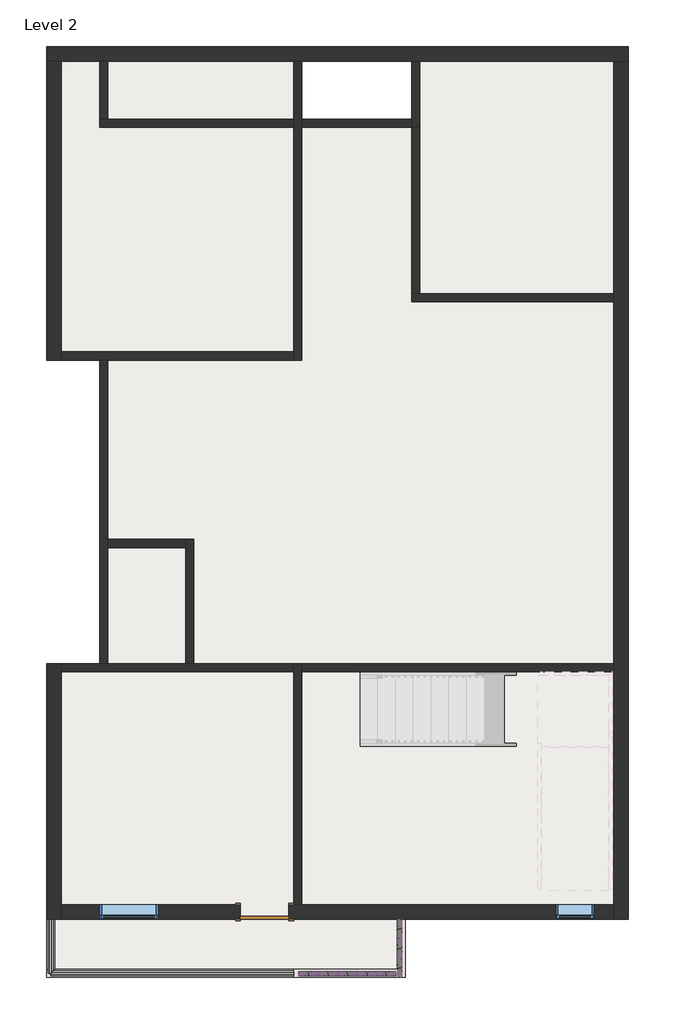
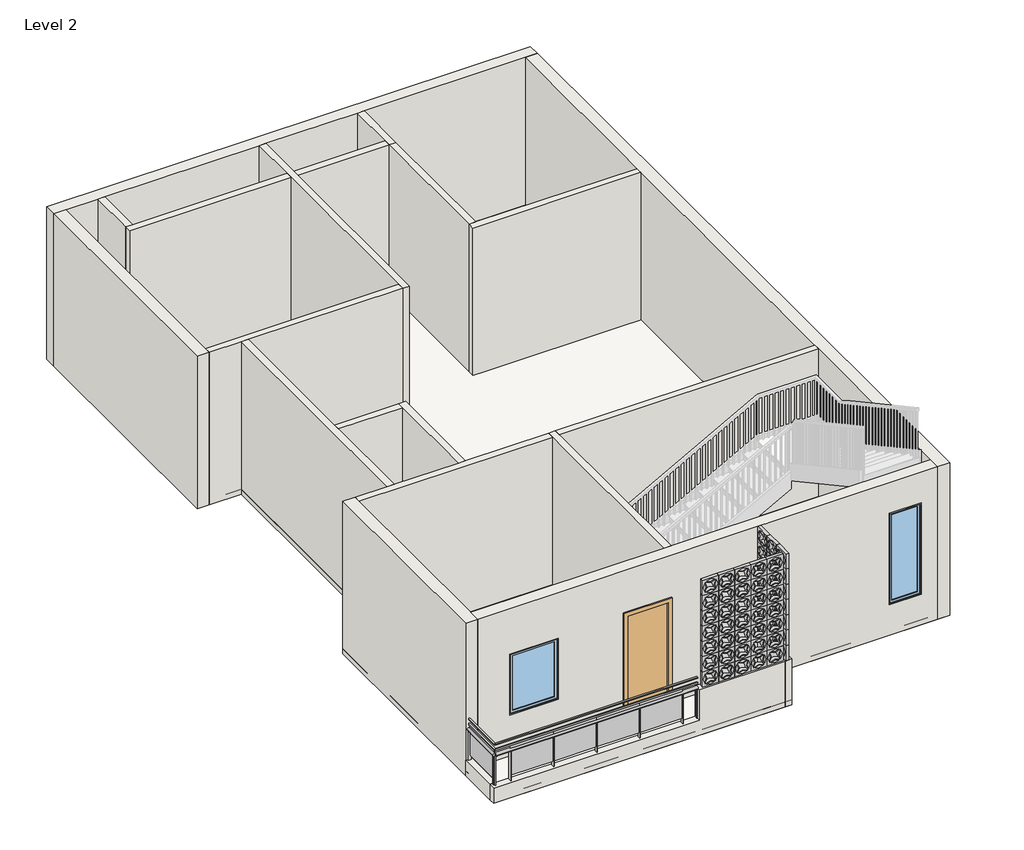
# One storey, part 1 of 2: 56 plates, 22 walls, 2 railings, 2 windows, 1 door, 1 roof.
"""IFC4 building model written with IfcOpenShell, lengths in millimetres."""

from ifc_helpers import new_model, si_unit, point, frame, origin, place, context, project, spatial, polyline, ellipse_curve, trimmed, outline, extrude, faceted_brep, transform, mapped, element, save
from ifc_brep_helpers import plane_surface, extruded_surface, advanced_brep
from components import door_5e1232af, plate_14329628, window_fc882ab3, fixed_4x3_c1f32544

model = new_model("IFC4")

# Units and contexts
model_context = context("Model", 3, world=origin())
ifc_project = project(units=[si_unit("LENGTHUNIT", "METRE", prefix="MILLI")], contexts=[model_context])

# Site, building, storey
site = spatial("IfcSite", under=ifc_project)
building = spatial("IfcBuilding", under=site)
storey = spatial("IfcBuildingStorey", under=building, Name="Level 2", Elevation=3048.0)

# Door
placement = place(None, origin())
door_shape = door_5e1232af(model_context)
element("IfcDoor", 1, ObjectType="Single-Flush : 30\" x 84\"", at=placement, inside=storey, context=model_context, shape_type="MappedRepresentation", body=[
    mapped(door_shape, transform((-1957.86646, -4503.4834702, 3048.0), x_axis=(1.0, 0.0, 0.0), y_axis=(0.0, 1.0, 0.0), z_axis=(0.0, 0.0, 1.0))),
])

# Plates
plate_shape = plate_14329628(model_context)
element("IfcPlate", 2, at=placement, inside=storey, context=model_context, shape_type="MappedRepresentation", body=[
    mapped(plate_shape, transform((194.78354, -4770.1834704, 3962.4), x_axis=(0.0, -1.0, 0.0), y_axis=(1.0, 0.0, 0.0), z_axis=(0.0, 0.0, 1.0))),
])
element("IfcPlate", 3, at=placement, inside=storey, context=model_context, shape_type="MappedRepresentation", body=[
    mapped(plate_shape, transform((194.78354, -5074.9834705, 3962.4), x_axis=(0.0, -1.0, 0.0), y_axis=(1.0, 0.0, 0.0), z_axis=(0.0, 0.0, 1.0))),
])
element("IfcPlate", 4, at=placement, inside=storey, context=model_context, shape_type="MappedRepresentation", body=[
    mapped(plate_shape, transform((194.78354, -5379.7834704, 3962.4), x_axis=(0.0, -1.0, 0.0), y_axis=(1.0, 0.0, 0.0), z_axis=(0.0, 0.0, 1.0))),
])
element("IfcPlate", 5, at=placement, inside=storey, context=model_context, shape_type="MappedRepresentation", body=[
    mapped(plate_shape, transform((194.78354, -4770.1834704, 4267.2), x_axis=(0.0, -1.0, 0.0), y_axis=(1.0, 0.0, 0.0), z_axis=(0.0, 0.0, 1.0))),
])
element("IfcPlate", 6, at=placement, inside=storey, context=model_context, shape_type="MappedRepresentation", body=[
    mapped(plate_shape, transform((194.78354, -5074.9834705, 4267.2), x_axis=(0.0, -1.0, 0.0), y_axis=(1.0, 0.0, 0.0), z_axis=(0.0, 0.0, 1.0))),
])
element("IfcPlate", 7, at=placement, inside=storey, context=model_context, shape_type="MappedRepresentation", body=[
    mapped(plate_shape, transform((194.78354, -5379.7834704, 4267.2), x_axis=(0.0, -1.0, 0.0), y_axis=(1.0, 0.0, 0.0), z_axis=(0.0, 0.0, 1.0))),
])
element("IfcPlate", 8, at=placement, inside=storey, context=model_context, shape_type="MappedRepresentation", body=[
    mapped(plate_shape, transform((194.78354, -4770.1834704, 4572.0), x_axis=(0.0, -1.0, 0.0), y_axis=(1.0, 0.0, 0.0), z_axis=(0.0, 0.0, 1.0))),
])
element("IfcPlate", 9, at=placement, inside=storey, context=model_context, shape_type="MappedRepresentation", body=[
    mapped(plate_shape, transform((194.78354, -5074.9834705, 4572.0), x_axis=(0.0, -1.0, 0.0), y_axis=(1.0, 0.0, 0.0), z_axis=(0.0, 0.0, 1.0))),
])
element("IfcPlate", 10, at=placement, inside=storey, context=model_context, shape_type="MappedRepresentation", body=[
    mapped(plate_shape, transform((194.78354, -5379.7834704, 4572.0), x_axis=(0.0, -1.0, 0.0), y_axis=(1.0, 0.0, 0.0), z_axis=(0.0, 0.0, 1.0))),
])
element("IfcPlate", 11, at=placement, inside=storey, context=model_context, shape_type="MappedRepresentation", body=[
    mapped(plate_shape, transform((194.78354, -4770.1834704, 4876.8), x_axis=(0.0, -1.0, 0.0), y_axis=(1.0, 0.0, 0.0), z_axis=(0.0, 0.0, 1.0))),
])
element("IfcPlate", 12, at=placement, inside=storey, context=model_context, shape_type="MappedRepresentation", body=[
    mapped(plate_shape, transform((194.78354, -5074.9834705, 4876.8), x_axis=(0.0, -1.0, 0.0), y_axis=(1.0, 0.0, 0.0), z_axis=(0.0, 0.0, 1.0))),
])
element("IfcPlate", 13, at=placement, inside=storey, context=model_context, shape_type="MappedRepresentation", body=[
    mapped(plate_shape, transform((194.78354, -5379.7834704, 4876.8), x_axis=(0.0, -1.0, 0.0), y_axis=(1.0, 0.0, 0.0), z_axis=(0.0, 0.0, 1.0))),
])
element("IfcPlate", 14, at=placement, inside=storey, context=model_context, shape_type="MappedRepresentation", body=[
    mapped(plate_shape, transform((194.78354, -4770.1834704, 5181.6), x_axis=(0.0, -1.0, 0.0), y_axis=(1.0, 0.0, 0.0), z_axis=(0.0, 0.0, 1.0))),
])
element("IfcPlate", 15, at=placement, inside=storey, context=model_context, shape_type="MappedRepresentation", body=[
    mapped(plate_shape, transform((194.78354, -5074.9834705, 5181.6), x_axis=(0.0, -1.0, 0.0), y_axis=(1.0, 0.0, 0.0), z_axis=(0.0, 0.0, 1.0))),
])
element("IfcPlate", 16, at=placement, inside=storey, context=model_context, shape_type="MappedRepresentation", body=[
    mapped(plate_shape, transform((194.78354, -5379.7834704, 5181.6), x_axis=(0.0, -1.0, 0.0), y_axis=(1.0, 0.0, 0.0), z_axis=(0.0, 0.0, 1.0))),
])
element("IfcPlate", 17, at=placement, inside=storey, context=model_context, shape_type="MappedRepresentation", body=[
    mapped(plate_shape, transform((194.78354, -4770.1834704, 5486.4), x_axis=(0.0, -1.0, 0.0), y_axis=(1.0, 0.0, 0.0), z_axis=(0.0, 0.0, 1.0))),
])
element("IfcPlate", 18, at=placement, inside=storey, context=model_context, shape_type="MappedRepresentation", body=[
    mapped(plate_shape, transform((194.78354, -5074.9834705, 5486.4), x_axis=(0.0, -1.0, 0.0), y_axis=(1.0, 0.0, 0.0), z_axis=(0.0, 0.0, 1.0))),
])
element("IfcPlate", 19, at=placement, inside=storey, context=model_context, shape_type="MappedRepresentation", body=[
    mapped(plate_shape, transform((194.78354, -5379.7834704, 5486.4), x_axis=(0.0, -1.0, 0.0), y_axis=(1.0, 0.0, 0.0), z_axis=(0.0, 0.0, 1.0))),
])
element("IfcPlate", 20, at=placement, inside=storey, context=model_context, shape_type="MappedRepresentation", body=[
    mapped(plate_shape, transform((194.78354, -4770.1834704, 5791.2), x_axis=(0.0, -1.0, 0.0), y_axis=(1.0, 0.0, 0.0), z_axis=(0.0, 0.0, 1.0))),
])
element("IfcPlate", 21, at=placement, inside=storey, context=model_context, shape_type="MappedRepresentation", body=[
    mapped(plate_shape, transform((194.78354, -5074.9834705, 5791.2), x_axis=(0.0, -1.0, 0.0), y_axis=(1.0, 0.0, 0.0), z_axis=(0.0, 0.0, 1.0))),
])
element("IfcPlate", 22, at=placement, inside=storey, context=model_context, shape_type="MappedRepresentation", body=[
    mapped(plate_shape, transform((194.78354, -5379.7834704, 5791.2), x_axis=(0.0, -1.0, 0.0), y_axis=(1.0, 0.0, 0.0), z_axis=(0.0, 0.0, 1.0))),
])
element("IfcPlate", 23, at=placement, inside=storey, context=model_context, shape_type="MappedRepresentation", body=[
    mapped(plate_shape, transform((-1272.0664598, -5443.2834702, 3962.4), x_axis=(1.0, 0.0, 0.0), y_axis=(0.0, 1.0, 0.0), z_axis=(0.0, 0.0, 1.0))),
])
element("IfcPlate", 24, at=placement, inside=storey, context=model_context, shape_type="MappedRepresentation", body=[
    mapped(plate_shape, transform((-967.2664597, -5443.2834702, 3962.4), x_axis=(1.0, 0.0, 0.0), y_axis=(0.0, 1.0, 0.0), z_axis=(0.0, 0.0, 1.0))),
])
element("IfcPlate", 25, at=placement, inside=storey, context=model_context, shape_type="MappedRepresentation", body=[
    mapped(plate_shape, transform((-662.4664597, -5443.2834702, 3962.4), x_axis=(1.0, 0.0, 0.0), y_axis=(0.0, 1.0, 0.0), z_axis=(0.0, 0.0, 1.0))),
])
element("IfcPlate", 26, at=placement, inside=storey, context=model_context, shape_type="MappedRepresentation", body=[
    mapped(plate_shape, transform((-1272.0664598, -5443.2834702, 4267.2), x_axis=(1.0, 0.0, 0.0), y_axis=(0.0, 1.0, 0.0), z_axis=(0.0, 0.0, 1.0))),
])
element("IfcPlate", 27, at=placement, inside=storey, context=model_context, shape_type="MappedRepresentation", body=[
    mapped(plate_shape, transform((-967.2664597, -5443.2834702, 4267.2), x_axis=(1.0, 0.0, 0.0), y_axis=(0.0, 1.0, 0.0), z_axis=(0.0, 0.0, 1.0))),
])
element("IfcPlate", 28, at=placement, inside=storey, context=model_context, shape_type="MappedRepresentation", body=[
    mapped(plate_shape, transform((-662.4664597, -5443.2834702, 4267.2), x_axis=(1.0, 0.0, 0.0), y_axis=(0.0, 1.0, 0.0), z_axis=(0.0, 0.0, 1.0))),
])
element("IfcPlate", 29, at=placement, inside=storey, context=model_context, shape_type="MappedRepresentation", body=[
    mapped(plate_shape, transform((-1272.0664598, -5443.2834702, 4572.0), x_axis=(1.0, 0.0, 0.0), y_axis=(0.0, 1.0, 0.0), z_axis=(0.0, 0.0, 1.0))),
])
element("IfcPlate", 30, at=placement, inside=storey, context=model_context, shape_type="MappedRepresentation", body=[
    mapped(plate_shape, transform((-967.2664597, -5443.2834702, 4572.0), x_axis=(1.0, 0.0, 0.0), y_axis=(0.0, 1.0, 0.0), z_axis=(0.0, 0.0, 1.0))),
])
element("IfcPlate", 31, at=placement, inside=storey, context=model_context, shape_type="MappedRepresentation", body=[
    mapped(plate_shape, transform((-662.4664597, -5443.2834702, 4572.0), x_axis=(1.0, 0.0, 0.0), y_axis=(0.0, 1.0, 0.0), z_axis=(0.0, 0.0, 1.0))),
])
element("IfcPlate", 32, at=placement, inside=storey, context=model_context, shape_type="MappedRepresentation", body=[
    mapped(plate_shape, transform((-1272.0664598, -5443.2834702, 4876.8), x_axis=(1.0, 0.0, 0.0), y_axis=(0.0, 1.0, 0.0), z_axis=(0.0, 0.0, 1.0))),
])
element("IfcPlate", 33, at=placement, inside=storey, context=model_context, shape_type="MappedRepresentation", body=[
    mapped(plate_shape, transform((-967.2664597, -5443.2834702, 4876.8), x_axis=(1.0, 0.0, 0.0), y_axis=(0.0, 1.0, 0.0), z_axis=(0.0, 0.0, 1.0))),
])
element("IfcPlate", 34, at=placement, inside=storey, context=model_context, shape_type="MappedRepresentation", body=[
    mapped(plate_shape, transform((-662.4664597, -5443.2834702, 4876.8), x_axis=(1.0, 0.0, 0.0), y_axis=(0.0, 1.0, 0.0), z_axis=(0.0, 0.0, 1.0))),
])
element("IfcPlate", 35, at=placement, inside=storey, context=model_context, shape_type="MappedRepresentation", body=[
    mapped(plate_shape, transform((-1272.0664598, -5443.2834702, 5181.6), x_axis=(1.0, 0.0, 0.0), y_axis=(0.0, 1.0, 0.0), z_axis=(0.0, 0.0, 1.0))),
])
element("IfcPlate", 36, at=placement, inside=storey, context=model_context, shape_type="MappedRepresentation", body=[
    mapped(plate_shape, transform((-967.2664597, -5443.2834702, 5181.6), x_axis=(1.0, 0.0, 0.0), y_axis=(0.0, 1.0, 0.0), z_axis=(0.0, 0.0, 1.0))),
])
element("IfcPlate", 37, at=placement, inside=storey, context=model_context, shape_type="MappedRepresentation", body=[
    mapped(plate_shape, transform((-662.4664597, -5443.2834702, 5181.6), x_axis=(1.0, 0.0, 0.0), y_axis=(0.0, 1.0, 0.0), z_axis=(0.0, 0.0, 1.0))),
])
element("IfcPlate", 38, at=placement, inside=storey, context=model_context, shape_type="MappedRepresentation", body=[
    mapped(plate_shape, transform((-1272.0664598, -5443.2834702, 5486.4), x_axis=(1.0, 0.0, 0.0), y_axis=(0.0, 1.0, 0.0), z_axis=(0.0, 0.0, 1.0))),
])
element("IfcPlate", 39, at=placement, inside=storey, context=model_context, shape_type="MappedRepresentation", body=[
    mapped(plate_shape, transform((-967.2664597, -5443.2834702, 5486.4), x_axis=(1.0, 0.0, 0.0), y_axis=(0.0, 1.0, 0.0), z_axis=(0.0, 0.0, 1.0))),
])
element("IfcPlate", 40, at=placement, inside=storey, context=model_context, shape_type="MappedRepresentation", body=[
    mapped(plate_shape, transform((-662.4664597, -5443.2834702, 5486.4), x_axis=(1.0, 0.0, 0.0), y_axis=(0.0, 1.0, 0.0), z_axis=(0.0, 0.0, 1.0))),
])
element("IfcPlate", 41, at=placement, inside=storey, context=model_context, shape_type="MappedRepresentation", body=[
    mapped(plate_shape, transform((-1272.0664598, -5443.2834702, 5791.2), x_axis=(1.0, 0.0, 0.0), y_axis=(0.0, 1.0, 0.0), z_axis=(0.0, 0.0, 1.0))),
])
element("IfcPlate", 42, at=placement, inside=storey, context=model_context, shape_type="MappedRepresentation", body=[
    mapped(plate_shape, transform((-967.2664597, -5443.2834702, 5791.2), x_axis=(1.0, 0.0, 0.0), y_axis=(0.0, 1.0, 0.0), z_axis=(0.0, 0.0, 1.0))),
])
element("IfcPlate", 43, at=placement, inside=storey, context=model_context, shape_type="MappedRepresentation", body=[
    mapped(plate_shape, transform((-662.4664597, -5443.2834702, 5791.2), x_axis=(1.0, 0.0, 0.0), y_axis=(0.0, 1.0, 0.0), z_axis=(0.0, 0.0, 1.0))),
])
element("IfcPlate", 44, at=placement, inside=storey, context=model_context, shape_type="MappedRepresentation", body=[
    mapped(plate_shape, transform((-357.6664597, -5443.2834702, 3962.4), x_axis=(1.0, 0.0, 0.0), y_axis=(0.0, 1.0, 0.0), z_axis=(0.0, 0.0, 1.0))),
])
element("IfcPlate", 45, at=placement, inside=storey, context=model_context, shape_type="MappedRepresentation", body=[
    mapped(plate_shape, transform((-357.6664597, -5443.2834702, 4267.2), x_axis=(1.0, 0.0, 0.0), y_axis=(0.0, 1.0, 0.0), z_axis=(0.0, 0.0, 1.0))),
])
element("IfcPlate", 46, at=placement, inside=storey, context=model_context, shape_type="MappedRepresentation", body=[
    mapped(plate_shape, transform((-357.6664597, -5443.2834702, 4572.0), x_axis=(1.0, 0.0, 0.0), y_axis=(0.0, 1.0, 0.0), z_axis=(0.0, 0.0, 1.0))),
])
element("IfcPlate", 47, at=placement, inside=storey, context=model_context, shape_type="MappedRepresentation", body=[
    mapped(plate_shape, transform((-357.6664597, -5443.2834702, 4876.8), x_axis=(1.0, 0.0, 0.0), y_axis=(0.0, 1.0, 0.0), z_axis=(0.0, 0.0, 1.0))),
])
element("IfcPlate", 48, at=placement, inside=storey, context=model_context, shape_type="MappedRepresentation", body=[
    mapped(plate_shape, transform((-357.6664597, -5443.2834702, 5181.6), x_axis=(1.0, 0.0, 0.0), y_axis=(0.0, 1.0, 0.0), z_axis=(0.0, 0.0, 1.0))),
])
element("IfcPlate", 49, at=placement, inside=storey, context=model_context, shape_type="MappedRepresentation", body=[
    mapped(plate_shape, transform((-357.6664597, -5443.2834702, 5486.4), x_axis=(1.0, 0.0, 0.0), y_axis=(0.0, 1.0, 0.0), z_axis=(0.0, 0.0, 1.0))),
])
element("IfcPlate", 50, at=placement, inside=storey, context=model_context, shape_type="MappedRepresentation", body=[
    mapped(plate_shape, transform((-357.6664597, -5443.2834702, 5791.2), x_axis=(1.0, 0.0, 0.0), y_axis=(0.0, 1.0, 0.0), z_axis=(0.0, 0.0, 1.0))),
])
element("IfcPlate", 51, at=placement, inside=storey, context=model_context, shape_type="MappedRepresentation", body=[
    mapped(plate_shape, transform((-52.8664598, -5443.2834702, 4267.2), x_axis=(1.0, 0.0, 0.0), y_axis=(0.0, 1.0, 0.0), z_axis=(0.0, 0.0, 1.0))),
])
element("IfcPlate", 52, at=placement, inside=storey, context=model_context, shape_type="MappedRepresentation", body=[
    mapped(plate_shape, transform((-52.8664598, -5443.2834702, 4572.0), x_axis=(1.0, 0.0, 0.0), y_axis=(0.0, 1.0, 0.0), z_axis=(0.0, 0.0, 1.0))),
])
element("IfcPlate", 53, at=placement, inside=storey, context=model_context, shape_type="MappedRepresentation", body=[
    mapped(plate_shape, transform((-52.8664598, -5443.2834702, 4876.8), x_axis=(1.0, 0.0, 0.0), y_axis=(0.0, 1.0, 0.0), z_axis=(0.0, 0.0, 1.0))),
])
element("IfcPlate", 54, at=placement, inside=storey, context=model_context, shape_type="MappedRepresentation", body=[
    mapped(plate_shape, transform((-52.8664598, -5443.2834702, 5791.2), x_axis=(1.0, 0.0, 0.0), y_axis=(0.0, 1.0, 0.0), z_axis=(0.0, 0.0, 1.0))),
])
element("IfcPlate", 55, at=placement, inside=storey, context=model_context, shape_type="MappedRepresentation", body=[
    mapped(plate_shape, transform((-52.8664598, -5443.2834702, 3962.4), x_axis=(1.0, 0.0, 0.0), y_axis=(0.0, 1.0, 0.0), z_axis=(0.0, 0.0, 1.0))),
])
element("IfcPlate", 56, at=placement, inside=storey, context=model_context, shape_type="MappedRepresentation", body=[
    mapped(plate_shape, transform((-52.8664598, -5443.2834702, 5181.6), x_axis=(1.0, 0.0, 0.0), y_axis=(0.0, 1.0, 0.0), z_axis=(0.0, 0.0, 1.0))),
])
element("IfcPlate", 57, at=placement, inside=storey, context=model_context, shape_type="MappedRepresentation", body=[
    mapped(plate_shape, transform((-52.8664598, -5443.2834702, 5486.4), x_axis=(1.0, 0.0, 0.0), y_axis=(0.0, 1.0, 0.0), z_axis=(0.0, 0.0, 1.0))),
])

# Railings
element("IfcRailing", 58, ObjectType="Glass Panel - Bottom Fill", at=placement, inside=storey, context=model_context, shape_type="SolidModel", body=[
    advanced_brep(
    [(-5285.26646, -4617.7834702, 3962.4), (-5361.46646, -4617.7834702, 3962.4), (-5285.26646, -5468.6834702, 3962.4), (-5361.46646, -5468.6834702, 3962.4)],
    [
        (0, 1, ellipse_curve(frame((-5323.36646, -4617.7834702, 3962.4), z_axis=(0.0, 1.0, 0.0), x_axis=(-1.0, 0.0, 0.0)), 38.1, 28.575)),
        (1, 0, ellipse_curve(frame((-5323.36646, -4617.7834702, 3962.4), z_axis=(0.0, 1.0, 0.0), x_axis=(-1.0, 0.0, 0.0)), 38.1, 28.575)),
        (2, 3, ellipse_curve(frame((-5323.36646, -5468.6834702, 3962.4), z_axis=(0.0, -1.0, 0.0), x_axis=(-1.0, 0.0, 0.0)), 38.1, 28.575)),
        (3, 2, ellipse_curve(frame((-5323.36646, -5468.6834702, 3962.4), z_axis=(0.0, -1.0, 0.0), x_axis=(-1.0, 0.0, 0.0)), 38.1, 28.575)),
        (0, 2),
        (3, 1),
    ],
    [
        plane_surface(frame((-5323.36646, -4617.7834702, 3962.4), z_axis=(0.0, 1.0, 0.0), x_axis=(0.0, 0.0, -1.0))),
        plane_surface(frame((-5323.36646, -5468.6834702, 3962.4), z_axis=(0.0, -1.0, 0.0), x_axis=(0.0, 0.0, -1.0))),
        extruded_surface(trimmed(ellipse_curve(frame((-5323.36646, -5468.6834702, 3962.4), z_axis=(0.0, 1.0, 0.0), x_axis=(-1.0, 0.0, 0.0)), 38.1, 28.575), [point((-5285.26646, -5468.6834702, 3962.4))], [point((-5361.46646, -5468.6834702, 3962.4))], True, "CARTESIAN"), (0.0, 850.8999999999996, 0.0), 850.8999999999996),
        extruded_surface(trimmed(ellipse_curve(frame((-5323.36646, -5468.6834702, 3962.4), z_axis=(0.0, 1.0, 0.0), x_axis=(-1.0, 0.0, 0.0)), 38.1, 28.575), [point((-5361.46646, -5468.6834702, 3962.4))], [point((-5285.26646, -5468.6834702, 3962.4))], True, "CARTESIAN"), (0.0, 850.8999999999996, 0.0), 850.8999999999996),
    ],
    [
        (0, [[1, 2]]),
        (1, [[3, 4]]),
        (2, [[-1, 5, -4, 6]]),
        (3, [[-2, -6, -3, -5]]),
    ],
),
    extrude(outline(polyline([(-5336.06646, -4617.7834702), (-5310.66646, -4617.7834702), (-5310.66646, -5468.6834702), (-5336.06646, -5468.6834702), (-5336.06646, -4617.7834702)])), frame((0.0, 0.0, 4152.9), z_axis=(0.0, 0.0, 1.0), x_axis=(1.0, 0.0, 0.0)), (0.0, 0.0, 1.0), 25.4),
    extrude(outline(polyline([(-5336.06646, -4617.7834702), (-5310.66646, -4617.7834702), (-5310.66646, -5468.6834702), (-5336.06646, -5468.6834702), (-5336.06646, -4617.7834702)])), frame((0.0, 0.0, 4051.3), z_axis=(0.0, 0.0, 1.0), x_axis=(1.0, 0.0, 0.0)), (0.0, 0.0, 1.0), 25.4),
    extrude(outline(polyline([(-5348.76646, -5443.2834702), (-5297.96646, -5443.2834702), (-5297.96646, -5455.9834702), (-5348.76646, -5455.9834702), (-5348.76646, -5443.2834702)])), frame((0.0, 0.0, 3352.8), z_axis=(0.0, 0.0, 1.0), x_axis=(1.0, 0.0, 0.0)), (0.0, 0.0, 1.0), 581.025),
    extrude(outline(polyline([(-5316.831303, -4636.8334702), (-5316.831303, -5449.6334702), (-5323.181303, -5449.6334702), (-5323.181303, -4636.8334702), (-5316.831303, -4636.8334702)])), frame((0.0, 0.0, 3454.4), z_axis=(0.0, 0.0, 1.0), x_axis=(1.0, 0.0, 0.0)), (0.0, 0.0, 1.0), 596.9),
    extrude(outline(polyline([(-5348.76646, -4630.4834702), (-5297.96646, -4630.4834702), (-5297.96646, -4643.1834702), (-5348.76646, -4643.1834702), (-5348.76646, -4630.4834702)])), frame((0.0, 0.0, 3352.8), z_axis=(0.0, 0.0, 1.0), x_axis=(1.0, 0.0, 0.0)), (0.0, 0.0, 1.0), 581.025),
    extrude(outline(polyline([(-5332.89146, -5455.9834702), (-5313.84146, -5455.9834702), (-5313.84146, -5475.0334702), (-5332.89146, -5475.0334702), (-5332.89146, -5455.9834702)])), frame((0.0, 0.0, 3352.8), z_axis=(0.0, 0.0, 1.0), x_axis=(1.0, 0.0, 0.0)), (0.0, 0.0, 1.0), 581.025),
    extrude(outline(polyline([(-5332.89146, -4611.4334702), (-5313.84146, -4611.4334702), (-5313.84146, -4630.4834702), (-5332.89146, -4630.4834702), (-5332.89146, -4611.4334702)])), frame((0.0, 0.0, 3352.8), z_axis=(0.0, 0.0, 1.0), x_axis=(1.0, 0.0, 0.0)), (0.0, 0.0, 1.0), 581.025),
])
element("IfcRailing", 59, ObjectType="Glass Panel - Bottom Fill", at=placement, inside=storey, context=model_context, shape_type="SolidModel", body=[
    advanced_brep(
    [(-1500.66646, -5506.7834702, 3962.4), (-1500.66646, -5430.5834702, 3962.4), (-5323.36646, -5506.7834702, 3962.4), (-5323.36646, -5430.5834702, 3962.4)],
    [
        (0, 1, ellipse_curve(frame((-1500.66646, -5468.6834702, 3962.4), z_axis=(1.0, 0.0, 0.0), x_axis=(0.0, 1.0, 0.0)), 38.1, 28.575)),
        (1, 0, ellipse_curve(frame((-1500.66646, -5468.6834702, 3962.4), z_axis=(1.0, 0.0, 0.0), x_axis=(0.0, 1.0, 0.0)), 38.1, 28.575)),
        (2, 3, ellipse_curve(frame((-5323.36646, -5468.6834702, 3962.4), z_axis=(-1.0, 0.0, 0.0), x_axis=(0.0, 1.0, 0.0)), 38.1, 28.575)),
        (3, 2, ellipse_curve(frame((-5323.36646, -5468.6834702, 3962.4), z_axis=(-1.0, 0.0, 0.0), x_axis=(0.0, 1.0, 0.0)), 38.1, 28.575)),
        (0, 2),
        (3, 1),
    ],
    [
        plane_surface(frame((-1500.66646, -5468.6834702, 3962.4), z_axis=(1.0, 0.0, 0.0), x_axis=(0.0, -1.0, 0.0))),
        plane_surface(frame((-5323.36646, -5468.6834702, 3962.4), z_axis=(-1.0, 0.0, 0.0), x_axis=(0.0, -1.0, 0.0))),
        extruded_surface(trimmed(ellipse_curve(frame((-5323.36646, -5468.6834702, 3962.4), z_axis=(1.0, 0.0, 0.0), x_axis=(0.0, 1.0, 0.0)), 38.1, 28.575), [point((-5323.36646, -5506.7834702, 3962.4))], [point((-5323.36646, -5430.5834702, 3962.4))], True, "CARTESIAN"), (3822.7000000000003, 0.0, 0.0), 3822.7000000000003),
        extruded_surface(trimmed(ellipse_curve(frame((-5323.36646, -5468.6834702, 3962.4), z_axis=(1.0, 0.0, 0.0), x_axis=(0.0, 1.0, 0.0)), 38.1, 28.575), [point((-5323.36646, -5430.5834702, 3962.4))], [point((-5323.36646, -5506.7834702, 3962.4))], True, "CARTESIAN"), (3822.7000000000003, 0.0, 0.0), 3822.7000000000003),
    ],
    [
        (0, [[1, 2]]),
        (1, [[3, 4]]),
        (2, [[-1, 5, -4, 6]]),
        (3, [[-2, -6, -3, -5]]),
    ],
),
    extrude(outline(polyline([(-1500.66646, -5455.9834702), (-1500.66646, -5481.3834702), (-5323.36646, -5481.3834702), (-5323.36646, -5455.9834702), (-1500.66646, -5455.9834702)])), frame((0.0, 0.0, 4152.9), z_axis=(0.0, 0.0, 1.0), x_axis=(1.0, 0.0, 0.0)), (0.0, 0.0, 1.0), 25.4),
    extrude(outline(polyline([(-1500.66646, -5455.9834702), (-1500.66646, -5481.3834702), (-5323.36646, -5481.3834702), (-5323.36646, -5455.9834702), (-1500.66646, -5455.9834702)])), frame((0.0, 0.0, 4051.3), z_axis=(0.0, 0.0, 1.0), x_axis=(1.0, 0.0, 0.0)), (0.0, 0.0, 1.0), 25.4),
    extrude(outline(polyline([(-5031.26646, -5443.2834702), (-5031.26646, -5494.0834702), (-5043.96646, -5494.0834702), (-5043.96646, -5443.2834702), (-5031.26646, -5443.2834702)])), frame((0.0, 0.0, 3352.8), z_axis=(0.0, 0.0, 1.0), x_axis=(1.0, 0.0, 0.0)), (0.0, 0.0, 1.0), 581.025),
    extrude(outline(polyline([(-4224.81646, -5475.2186272), (-5037.61646, -5475.2186272), (-5037.61646, -5468.8686272), (-4224.81646, -5468.8686272), (-4224.81646, -5475.2186272)])), frame((0.0, 0.0, 3454.4), z_axis=(0.0, 0.0, 1.0), x_axis=(1.0, 0.0, 0.0)), (0.0, 0.0, 1.0), 596.9),
    extrude(outline(polyline([(-4218.46646, -5443.2834702), (-4218.46646, -5494.0834702), (-4231.16646, -5494.0834702), (-4231.16646, -5443.2834702), (-4218.46646, -5443.2834702)])), frame((0.0, 0.0, 3352.8), z_axis=(0.0, 0.0, 1.0), x_axis=(1.0, 0.0, 0.0)), (0.0, 0.0, 1.0), 581.025),
    extrude(outline(polyline([(-3412.01646, -5475.2186272), (-4224.81646, -5475.2186272), (-4224.81646, -5468.8686272), (-3412.01646, -5468.8686272), (-3412.01646, -5475.2186272)])), frame((0.0, 0.0, 3454.4), z_axis=(0.0, 0.0, 1.0), x_axis=(1.0, 0.0, 0.0)), (0.0, 0.0, 1.0), 596.9),
    extrude(outline(polyline([(-3405.66646, -5443.2834702), (-3405.66646, -5494.0834702), (-3418.36646, -5494.0834702), (-3418.36646, -5443.2834702), (-3405.66646, -5443.2834702)])), frame((0.0, 0.0, 3352.8), z_axis=(0.0, 0.0, 1.0), x_axis=(1.0, 0.0, 0.0)), (0.0, 0.0, 1.0), 581.025),
    extrude(outline(polyline([(-2599.21646, -5475.2186272), (-3412.01646, -5475.2186272), (-3412.01646, -5468.8686272), (-2599.21646, -5468.8686272), (-2599.21646, -5475.2186272)])), frame((0.0, 0.0, 3454.4), z_axis=(0.0, 0.0, 1.0), x_axis=(1.0, 0.0, 0.0)), (0.0, 0.0, 1.0), 596.9),
    extrude(outline(polyline([(-2592.86646, -5443.2834702), (-2592.86646, -5494.0834702), (-2605.56646, -5494.0834702), (-2605.56646, -5443.2834702), (-2592.86646, -5443.2834702)])), frame((0.0, 0.0, 3352.8), z_axis=(0.0, 0.0, 1.0), x_axis=(1.0, 0.0, 0.0)), (0.0, 0.0, 1.0), 581.025),
    extrude(outline(polyline([(-1786.41646, -5475.2186272), (-2599.21646, -5475.2186272), (-2599.21646, -5468.8686272), (-1786.41646, -5468.8686272), (-1786.41646, -5475.2186272)])), frame((0.0, 0.0, 3454.4), z_axis=(0.0, 0.0, 1.0), x_axis=(1.0, 0.0, 0.0)), (0.0, 0.0, 1.0), 596.9),
    extrude(outline(polyline([(-1780.06646, -5443.2834702), (-1780.06646, -5494.0834702), (-1792.76646, -5494.0834702), (-1792.76646, -5443.2834702), (-1780.06646, -5443.2834702)])), frame((0.0, 0.0, 3352.8), z_axis=(0.0, 0.0, 1.0), x_axis=(1.0, 0.0, 0.0)), (0.0, 0.0, 1.0), 581.025),
    extrude(outline(polyline([(-5310.66646, -5459.1584702), (-5310.66646, -5478.2084702), (-5329.71646, -5478.2084702), (-5329.71646, -5459.1584702), (-5310.66646, -5459.1584702)])), frame((0.0, 0.0, 3352.8), z_axis=(0.0, 0.0, 1.0), x_axis=(1.0, 0.0, 0.0)), (0.0, 0.0, 1.0), 581.025),
    extrude(outline(polyline([(-1494.31646, -5459.1584702), (-1494.31646, -5478.2084702), (-1513.36646, -5478.2084702), (-1513.36646, -5459.1584702), (-1494.31646, -5459.1584702)])), frame((0.0, 0.0, 3352.8), z_axis=(0.0, 0.0, 1.0), x_axis=(1.0, 0.0, 0.0)), (0.0, 0.0, 1.0), 581.025),
])

# Roof
element("IfcRoof", 60, ObjectType="Generic - 4\"", at=placement, inside=storey, context=model_context, shape_type="Brep", body=[
    faceted_brep([(-5386.86646, 4170.6165298, 3048.0), (-5386.86646, 9098.2165298, 3048.0), (3757.13354, 9098.2165298, 3048.0), (3757.13354, -4617.7834702, 3048.0), (251.93354, -4617.7834702, 3048.0), (251.93354, -5532.1834702, 3048.0), (-5386.86646, -5532.1834702, 3048.0), (-5386.86646, -604.5834702, 3048.0), (-5158.26646, -604.5834702, 3048.0), (-4548.66646, -604.5834702, 3048.0), (-4548.66646, 4170.6165298, 3048.0), (-5158.26646, 4170.6165298, 3048.0), (353.53354, 8869.6165298, 3048.0), (-1373.66646, 8869.6165298, 3048.0), (-1373.66646, 7955.2165298, 3048.0), (353.53354, 7955.2165298, 3048.0), (3757.13354, -4617.7834702, 3149.6), (3757.13354, 9098.2165298, 3149.6), (-5386.86646, 9098.2165298, 3149.6), (-5386.86646, 4170.6165298, 3149.6), (-5158.26646, 4170.6165298, 3149.6), (-4548.66646, 4170.6165298, 3149.6), (-4548.66646, -604.5834702, 3149.6), (-5158.26646, -604.5834702, 3149.6), (-5386.86646, -604.5834702, 3149.6), (-5386.86646, -5532.1834702, 3149.6), (251.93354, -5532.1834702, 3149.6), (251.93354, -4617.7834702, 3149.6), (-1373.66646, 8869.6165298, 3149.6), (353.53354, 8869.6165298, 3149.6), (353.53354, 7955.2165298, 3149.6), (-1373.66646, 7955.2165298, 3149.6)], [[[0, 1, 2, 3, 4, 5, 6, 7, 8, 9, 10, 11], [12, 13, 14, 15]], [[16, 17, 18, 19, 20, 21, 22, 23, 24, 25, 26, 27], [28, 29, 30, 31]], [[2, 1, 18, 17]], [[1, 0, 19, 18]], [[3, 2, 17, 16]], [[4, 3, 16, 27]], [[5, 4, 27, 26]], [[6, 5, 26, 25]], [[12, 29, 28, 13]], [[13, 28, 31, 14]], [[14, 31, 30, 15]], [[29, 12, 15, 30]], [[22, 9, 8, 7, 24, 23]], [[10, 9, 22, 21]], [[19, 0, 11, 10, 21, 20]], [[7, 6, 25, 24]]]),
])

# Walls
element("IfcWall", 61, ObjectType="Generic - 5\"", at=placement, inside=storey, context=model_context, shape_type="Brep", body=[
    faceted_brep([(-1500.66646, -604.5834702, 3048.0), (-3075.46646, -604.5834702, 3048.0), (-3202.46646, -604.5834702, 3048.0), (-4421.66646, -604.5834702, 3048.0), (-4548.66646, -604.5834702, 3048.0), (-5158.26646, -604.5834702, 3048.0), (-5158.26646, -604.5834702, 6096.0), (-4548.66646, -604.5834702, 6096.0), (-4421.66646, -604.5834702, 6096.0), (-3202.46646, -604.5834702, 6096.0), (-3075.46646, -604.5834702, 6096.0), (-1500.66646, -604.5834702, 6096.0), (-1500.66646, -731.5834702, 3048.0), (-1500.66646, -731.5834702, 6096.0), (-5158.26646, -731.5834702, 6096.0), (-5158.26646, -731.5834702, 3048.0)], [[[0, 1, 2, 3, 4, 5, 6, 7, 8, 9, 10, 11]], [[12, 13, 14, 15]], [[5, 4, 3, 2, 1, 0, 12, 15]], [[11, 10, 9, 8, 7, 6, 14, 13]], [[0, 11, 13, 12]], [[6, 5, 15, 14]]]),
])
element("IfcWall", 62, ObjectType="Generic - 5\"", at=placement, inside=storey, context=model_context, shape_type="SweptSolid", body=[
    extrude(outline(polyline([(3528.53354, -731.5834702), (-1373.66646, -731.5834702), (-1373.66646, -604.5834702), (3528.53354, -604.5834702), (3528.53354, -731.5834702)])), frame((0.0, 0.0, 3048.0), z_axis=(0.0, 0.0, 1.0), x_axis=(1.0, 0.0, 0.0)), (0.0, 0.0, 1.0), 3048.0),
])
element("IfcWall", 63, ObjectType="Generic - 5\"", at=placement, inside=storey, context=model_context, shape_type="Brep", body=[
    faceted_brep([(-1500.66646, 8869.6165298, 3048.0), (-1500.66646, 7955.2165298, 3048.0), (-1500.66646, 7828.2165298, 3048.0), (-1500.66646, 4297.6165298, 3048.0), (-1500.66646, 4170.6165298, 3048.0), (-1500.66646, 4170.6165298, 6096.0), (-1500.66646, 4297.6165298, 6096.0), (-1500.66646, 7828.2165298, 6096.0), (-1500.66646, 7955.2165298, 6096.0), (-1500.66646, 8869.6165298, 6096.0), (-1373.66646, 8869.6165298, 3048.0), (-1373.66646, 8869.6165298, 6096.0), (-1373.66646, 7955.2165298, 6096.0), (-1373.66646, 7828.2165298, 6096.0), (-1373.66646, 4170.6165298, 6096.0), (-1373.66646, 4170.6165298, 3048.0), (-1373.66646, 7828.2165298, 3048.0), (-1373.66646, 7955.2165298, 3048.0)], [[[0, 1, 2, 3, 4, 5, 6, 7, 8, 9]], [[10, 11, 12, 13, 14, 15, 16, 17]], [[4, 3, 2, 1, 0, 10, 17, 16, 15]], [[9, 8, 7, 6, 5, 14, 13, 12, 11]], [[0, 9, 11, 10]], [[5, 4, 15, 14]]]),
])
element("IfcWall", 64, ObjectType="Generic - 5\"", at=placement, inside=storey, context=model_context, shape_type="Brep", body=[
    faceted_brep([(-1500.66646, 4297.6165298, 3048.0), (-5158.26646, 4297.6165298, 3048.0), (-5158.26646, 4297.6165298, 6096.0), (-1500.66646, 4297.6165298, 6096.0), (-1500.66646, 4170.6165298, 3048.0), (-1500.66646, 4170.6165298, 6096.0), (-4421.66646, 4170.6165298, 6096.0), (-4548.66646, 4170.6165298, 6096.0), (-5158.26646, 4170.6165298, 6096.0), (-5158.26646, 4170.6165298, 3048.0), (-4548.66646, 4170.6165298, 3048.0), (-4421.66646, 4170.6165298, 3048.0)], [[[0, 1, 2, 3]], [[4, 5, 6, 7, 8, 9, 10, 11]], [[1, 0, 4, 11, 10, 9]], [[3, 2, 8, 7, 6, 5]], [[0, 3, 5, 4]], [[2, 1, 9, 8]]]),
])
element("IfcWall", 65, ObjectType="Generic - 5\"", at=placement, inside=storey, context=model_context, shape_type="Brep", body=[
    faceted_brep([(353.53354, 8869.6165298, 3048.0), (353.53354, 7955.2165298, 3048.0), (353.53354, 7828.2165298, 3048.0), (353.53354, 7828.2165298, 6096.0), (353.53354, 7955.2165298, 6096.0), (353.53354, 8869.6165298, 6096.0), (480.53354, 8869.6165298, 3048.0), (480.53354, 8869.6165298, 6096.0), (480.53354, 7828.2165298, 6096.0), (480.53354, 7828.2165298, 3048.0)], [[[0, 1, 2, 3, 4, 5]], [[6, 7, 8, 9]], [[2, 1, 0, 6, 9]], [[5, 4, 3, 8, 7]], [[0, 5, 7, 6]], [[3, 2, 9, 8]]]),
])
element("IfcWall", 66, ObjectType="Generic - 5\"", at=placement, inside=storey, context=model_context, shape_type="SweptSolid", body=[
    extrude(outline(polyline([(-1373.66646, 7955.2165298), (353.53354, 7955.2165298), (353.53354, 7828.2165298), (-1373.66646, 7828.2165298), (-1373.66646, 7955.2165298)])), frame((0.0, 0.0, 3048.0), z_axis=(0.0, 0.0, 1.0), x_axis=(1.0, 0.0, 0.0)), (0.0, 0.0, 1.0), 3048.0),
])
element("IfcWall", 67, ObjectType="Generic - 5\"", at=placement, inside=storey, context=model_context, shape_type="Brep", body=[
    faceted_brep([(3528.53354, 5212.0165298, 3048.0), (480.53354, 5212.0165298, 3048.0), (353.53354, 5212.0165298, 3048.0), (353.53354, 5212.0165298, 6096.0), (480.53354, 5212.0165298, 6096.0), (3528.53354, 5212.0165298, 6096.0), (3528.53354, 5085.0165298, 3048.0), (3528.53354, 5085.0165298, 6096.0), (353.53354, 5085.0165298, 6096.0), (353.53354, 5085.0165298, 3048.0)], [[[0, 1, 2, 3, 4, 5]], [[6, 7, 8, 9]], [[2, 1, 0, 6, 9]], [[5, 4, 3, 8, 7]], [[0, 5, 7, 6]], [[3, 2, 9, 8]]]),
])
element("IfcWall", 68, ObjectType="Generic - 5\"", at=placement, inside=storey, context=model_context, shape_type="SweptSolid", body=[
    extrude(outline(polyline([(480.53354, 7828.2165298), (480.53354, 5212.0165298), (353.53354, 5212.0165298), (353.53354, 7828.2165298), (480.53354, 7828.2165298)])), frame((0.0, 0.0, 3048.0), z_axis=(0.0, 0.0, 1.0), x_axis=(1.0, 0.0, 0.0)), (0.0, 0.0, 1.0), 3048.0),
])
element("IfcWall", 69, ObjectType="Generic - 5\"", at=placement, inside=storey, context=model_context, shape_type="Brep", body=[
    faceted_brep([(-4421.66646, -604.5834702, 3048.0), (-4421.66646, 1224.2165298, 3048.0), (-4421.66646, 1351.2165298, 3048.0), (-4421.66646, 4170.6165298, 3048.0), (-4421.66646, 4170.6165298, 6096.0), (-4421.66646, 1351.2165298, 6096.0), (-4421.66646, 1224.2165298, 6096.0), (-4421.66646, -604.5834702, 6096.0), (-4548.66646, -604.5834702, 3048.0), (-4548.66646, -604.5834702, 6096.0), (-4548.66646, 4170.6165298, 6096.0), (-4548.66646, 4170.6165298, 3048.0)], [[[0, 1, 2, 3, 4, 5, 6, 7]], [[8, 9, 10, 11]], [[3, 2, 1, 0, 8, 11]], [[7, 6, 5, 4, 10, 9]], [[0, 7, 9, 8]], [[4, 3, 11, 10]]]),
])
element("IfcWall", 70, ObjectType="Generic - 5\"", at=placement, inside=storey, context=model_context, shape_type="Brep", body=[
    faceted_brep([(-3075.46646, -604.5834702, 3048.0), (-3075.46646, 1351.2165298, 3048.0), (-3075.46646, 1351.2165298, 6096.0), (-3075.46646, -604.5834702, 6096.0), (-3202.46646, -604.5834702, 3048.0), (-3202.46646, -604.5834702, 6096.0), (-3202.46646, 1224.2165298, 6096.0), (-3202.46646, 1351.2165298, 6096.0), (-3202.46646, 1351.2165298, 3048.0), (-3202.46646, 1224.2165298, 3048.0)], [[[0, 1, 2, 3]], [[4, 5, 6, 7, 8, 9]], [[1, 0, 4, 9, 8]], [[3, 2, 7, 6, 5]], [[0, 3, 5, 4]], [[2, 1, 8, 7]]]),
])
element("IfcWall", 71, ObjectType="Generic - 5\"", at=placement, inside=storey, context=model_context, shape_type="SweptSolid", body=[
    extrude(outline(polyline([(-4421.66646, 1351.2165298), (-3202.46646, 1351.2165298), (-3202.46646, 1224.2165298), (-4421.66646, 1224.2165298), (-4421.66646, 1351.2165298)])), frame((0.0, 0.0, 3048.0), z_axis=(0.0, 0.0, 1.0), x_axis=(1.0, 0.0, 0.0)), (0.0, 0.0, 1.0), 3048.0),
])
element("IfcWall", 72, ObjectType="Generic - 5\"", at=placement, inside=storey, context=model_context, shape_type="Brep", body=[
    faceted_brep([(-1500.66646, 7955.2165298, 3048.0), (-4421.66646, 7955.2165298, 3048.0), (-4548.66646, 7955.2165298, 3048.0), (-4548.66646, 7955.2165298, 6096.0), (-4421.66646, 7955.2165298, 6096.0), (-1500.66646, 7955.2165298, 6096.0), (-1500.66646, 7828.2165298, 3048.0), (-1500.66646, 7828.2165298, 6096.0), (-4548.66646, 7828.2165298, 6096.0), (-4548.66646, 7828.2165298, 3048.0)], [[[0, 1, 2, 3, 4, 5]], [[6, 7, 8, 9]], [[2, 1, 0, 6, 9]], [[5, 4, 3, 8, 7]], [[0, 5, 7, 6]], [[3, 2, 9, 8]]]),
])
element("IfcWall", 73, ObjectType="Generic - 5\"", at=placement, inside=storey, context=model_context, shape_type="SweptSolid", body=[
    extrude(outline(polyline([(-4421.66646, 8869.6165298), (-4421.66646, 7955.2165298), (-4548.66646, 7955.2165298), (-4548.66646, 8869.6165298), (-4421.66646, 8869.6165298)])), frame((0.0, 0.0, 3048.0), z_axis=(0.0, 0.0, 1.0), x_axis=(1.0, 0.0, 0.0)), (0.0, 0.0, 1.0), 3048.0),
])
element("IfcWall", 74, ObjectType="Generic - 5\"", at=placement, inside=storey, context=model_context, shape_type="Brep", body=[
    faceted_brep([(-1373.66646, -4389.1834702, 3048.0), (-1373.66646, -731.5834702, 3048.0), (-1373.66646, -604.5834702, 3048.0), (-1373.66646, -604.5834702, 6096.0), (-1373.66646, -731.5834702, 6096.0), (-1373.66646, -4389.1834702, 6096.0), (-1500.66646, -4389.1834702, 3048.0), (-1500.66646, -4389.1834702, 6096.0), (-1500.66646, -731.5834702, 6096.0), (-1500.66646, -604.5834702, 6096.0), (-1500.66646, -604.5834702, 3048.0), (-1500.66646, -731.5834702, 3048.0)], [[[0, 1, 2, 3, 4, 5]], [[6, 7, 8, 9, 10, 11]], [[2, 1, 0, 6, 11, 10]], [[5, 4, 3, 9, 8, 7]], [[3, 2, 10, 9]], [[0, 5, 7, 6]]]),
])
element("IfcWall", 75, ObjectType="Generic - 5\"", at=placement, inside=storey, context=model_context, shape_type="Brep", body=[
    faceted_brep([(124.93354, -4617.7834702, 3048.0), (124.93354, -5405.1834702, 3048.0), (124.93354, -5532.1834702, 3048.0), (124.93354, -5532.1834702, 3962.4), (124.93354, -5405.1834702, 3962.4), (124.93354, -4617.7834702, 3962.4), (251.93354, -4617.7834702, 3048.0), (251.93354, -4617.7834702, 3962.4), (251.93354, -5532.1834702, 3962.4), (251.93354, -5532.1834702, 3048.0)], [[[0, 1, 2, 3, 4, 5]], [[6, 7, 8, 9]], [[2, 1, 0, 6, 9]], [[5, 4, 3, 8, 7]], [[0, 5, 7, 6]], [[3, 2, 9, 8]]]),
])
element("IfcWall", 76, ObjectType="Generic - 5\"", at=placement, inside=storey, context=model_context, shape_type="Brep", body=[
    faceted_brep([(124.93354, -5405.1834702, 3048.0), (-5259.86646, -5405.1834702, 3048.0), (-5386.86646, -5405.1834702, 3048.0), (-5386.86646, -5405.1834702, 3352.8), (-5259.86646, -5405.1834702, 3352.8), (-1500.66646, -5405.1834702, 3352.8), (-1500.66646, -5405.1834702, 3962.4), (124.93354, -5405.1834702, 3962.4), (124.93354, -5532.1834702, 3048.0), (124.93354, -5532.1834702, 3962.4), (-1500.66646, -5532.1834702, 3962.4), (-1500.66646, -5532.1834702, 3352.8), (-5386.86646, -5532.1834702, 3352.8), (-5386.86646, -5532.1834702, 3048.0)], [[[0, 1, 2, 3, 4, 5, 6, 7]], [[8, 9, 10, 11, 12, 13]], [[0, 7, 9, 8]], [[3, 2, 13, 12]], [[2, 1, 0, 8, 13]], [[5, 4, 3, 12, 11]], [[6, 5, 11, 10]], [[7, 6, 10, 9]]]),
])
element("IfcWall", 77, ObjectType="Generic - 5\"", at=placement, inside=storey, context=model_context, shape_type="SweptSolid", body=[
    extrude(outline(polyline([(-5259.86646, -4617.7834702), (-5259.86646, -5405.1834702), (-5386.86646, -5405.1834702), (-5386.86646, -4617.7834702), (-5259.86646, -4617.7834702)])), frame((0.0, 0.0, 3048.0), z_axis=(0.0, 0.0, 1.0), x_axis=(1.0, 0.0, 0.0)), (0.0, 0.0, 1.0), 304.8),
])
element("IfcWall", 78, ObjectType="Generic -9\"", at=placement, inside=storey, context=model_context, shape_type="Brep", body=[
    faceted_brep([(-5386.86646, 8869.6165298, 3048.0), (-5158.26646, 8869.6165298, 3048.0), (-4548.66646, 8869.6165298, 3048.0), (-4421.66646, 8869.6165298, 3048.0), (-1500.66646, 8869.6165298, 3048.0), (-1373.66646, 8869.6165298, 3048.0), (353.53354, 8869.6165298, 3048.0), (480.53354, 8869.6165298, 3048.0), (3528.53354, 8869.6165298, 3048.0), (3757.13354, 8869.6165298, 3048.0), (3757.13354, 8869.6165298, 6096.0), (3528.53354, 8869.6165298, 6096.0), (480.53354, 8869.6165298, 6096.0), (353.53354, 8869.6165298, 6096.0), (-1373.66646, 8869.6165298, 6096.0), (-1500.66646, 8869.6165298, 6096.0), (-4421.66646, 8869.6165298, 6096.0), (-4548.66646, 8869.6165298, 6096.0), (-5158.26646, 8869.6165298, 6096.0), (-5386.86646, 8869.6165298, 6096.0), (-5386.86646, 9098.2165298, 3048.0), (-5386.86646, 9098.2165298, 6096.0), (3757.13354, 9098.2165298, 6096.0), (3757.13354, 9098.2165298, 3048.0)], [[[0, 1, 2, 3, 4, 5, 6, 7, 8, 9, 10, 11, 12, 13, 14, 15, 16, 17, 18, 19]], [[20, 21, 22, 23]], [[9, 8, 7, 6, 5, 4, 3, 2, 1, 0, 20, 23]], [[19, 18, 17, 16, 15, 14, 13, 12, 11, 10, 22, 21]], [[10, 9, 23, 22]], [[0, 19, 21, 20]]]),
])
element("IfcWall", 79, ObjectType="Generic -9\"", at=placement, inside=storey, context=model_context, shape_type="Brep", body=[
    faceted_brep([(3528.53354, 8869.6165298, 3048.0), (3528.53354, 5212.0165298, 3048.0), (3528.53354, 5085.0165298, 3048.0), (3528.53354, -604.5834702, 3048.0), (3528.53354, -731.5834702, 3048.0), (3528.53354, -4389.1834702, 3048.0), (3528.53354, -4617.7834702, 3048.0), (3528.53354, -4617.7834702, 6096.0), (3528.53354, -4389.1834702, 6096.0), (3528.53354, -731.5834702, 6096.0), (3528.53354, -604.5834702, 6096.0), (3528.53354, 5085.0165298, 6096.0), (3528.53354, 5212.0165298, 6096.0), (3528.53354, 8869.6165298, 6096.0), (3757.13354, 8869.6165298, 3048.0), (3757.13354, 8869.6165298, 6096.0), (3757.13354, -4617.7834702, 6096.0), (3757.13354, -4617.7834702, 3048.0)], [[[0, 1, 2, 3, 4, 5, 6, 7, 8, 9, 10, 11, 12, 13]], [[14, 15, 16, 17]], [[6, 5, 4, 3, 2, 1, 0, 14, 17]], [[13, 12, 11, 10, 9, 8, 7, 16, 15]], [[0, 13, 15, 14]], [[7, 6, 17, 16]]]),
])
element("IfcWall", 80, ObjectType="Generic -9\"", at=placement, inside=storey, context=model_context, shape_type="Brep", body=[
    faceted_brep([(3528.53354, -4389.1834702, 3048.0), (-1373.66646, -4389.1834702, 3048.0), (-1500.66646, -4389.1834702, 3048.0), (-1576.86646, -4389.1834702, 3048.0), (-1576.86646, -4389.1834702, 5181.6), (-2338.86646, -4389.1834702, 5181.6), (-2338.86646, -4389.1834702, 3048.0), (-5158.26646, -4389.1834702, 3048.0), (-5158.26646, -4389.1834702, 6096.0), (-1500.66646, -4389.1834702, 6096.0), (-1373.66646, -4389.1834702, 6096.0), (3528.53354, -4389.1834702, 6096.0), (2614.13354, -4389.1834702, 5486.4), (2614.13354, -4389.1834702, 3657.6), (3223.73354, -4389.1834702, 3657.6), (3223.73354, -4389.1834702, 5486.4), (-4548.66646, -4389.1834702, 5181.6), (-4548.66646, -4389.1834702, 3962.4), (-3634.26646, -4389.1834702, 3962.4), (-3634.26646, -4389.1834702, 5181.6), (-1576.86646, -4617.7834702, 5181.6), (-1576.86646, -4617.7834702, 3048.0), (124.93354, -4617.7834702, 3048.0), (251.93354, -4617.7834702, 3048.0), (3528.53354, -4617.7834702, 3048.0), (3528.53354, -4617.7834702, 6096.0), (-5158.26646, -4617.7834702, 6096.0), (-5158.26646, -4617.7834702, 3048.0), (-2338.86646, -4617.7834702, 3048.0), (-2338.86646, -4617.7834702, 5181.6), (2614.13354, -4617.7834702, 5486.4), (3223.73354, -4617.7834702, 5486.4), (3223.73354, -4617.7834702, 3657.6), (2614.13354, -4617.7834702, 3657.6), (-4548.66646, -4617.7834702, 5181.6), (-3634.26646, -4617.7834702, 5181.6), (-3634.26646, -4617.7834702, 3962.4), (-4548.66646, -4617.7834702, 3962.4)], [[[0, 1, 2, 3, 4, 5, 6, 7, 8, 9, 10, 11], [12, 13, 14, 15], [16, 17, 18, 19]], [[20, 21, 22, 23, 24, 25, 26, 27, 28, 29], [30, 31, 32, 33], [34, 35, 36, 37]], [[28, 27, 7, 6]], [[24, 23, 22, 21, 3, 2, 1, 0]], [[11, 10, 9, 8, 26, 25]], [[0, 11, 25, 24]], [[13, 12, 30, 33]], [[14, 13, 33, 32]], [[15, 14, 32, 31]], [[12, 15, 31, 30]], [[7, 27, 26, 8]], [[4, 3, 21, 20]], [[5, 4, 20, 29]], [[6, 5, 29, 28]], [[17, 16, 34, 37]], [[18, 17, 37, 36]], [[19, 18, 36, 35]], [[16, 19, 35, 34]]]),
])
element("IfcWall", 81, ObjectType="Generic -9\"", at=placement, inside=storey, context=model_context, shape_type="Brep", body=[
    faceted_brep([(-5158.26646, 4170.6165298, 3048.0), (-5158.26646, 4297.6165298, 3048.0), (-5158.26646, 8869.6165298, 3048.0), (-5158.26646, 8869.6165298, 6096.0), (-5158.26646, 4297.6165298, 6096.0), (-5158.26646, 4170.6165298, 6096.0), (-5386.86646, 4170.6165298, 3048.0), (-5386.86646, 4170.6165298, 6096.0), (-5386.86646, 8869.6165298, 6096.0), (-5386.86646, 8869.6165298, 3048.0)], [[[0, 1, 2, 3, 4, 5]], [[6, 7, 8, 9]], [[2, 1, 0, 6, 9]], [[5, 4, 3, 8, 7]], [[0, 5, 7, 6]], [[3, 2, 9, 8]]]),
])
element("IfcWall", 82, ObjectType="Generic -9\"", at=placement, inside=storey, context=model_context, shape_type="Brep", body=[
    faceted_brep([(-5158.26646, -4617.7834702, 6096.0), (-5158.26646, -4617.7834702, 3048.0), (-5158.26646, -4389.1834702, 3048.0), (-5158.26646, -731.5834702, 3048.0), (-5158.26646, -604.5834702, 3048.0), (-5158.26646, -604.5834702, 6096.0), (-5158.26646, -731.5834702, 6096.0), (-5158.26646, -4389.1834702, 6096.0), (-5386.86646, -4617.7834702, 3048.0), (-5386.86646, -4617.7834702, 3352.8), (-5386.86646, -4617.7834702, 6096.0), (-5386.86646, -604.5834702, 6096.0), (-5386.86646, -604.5834702, 3048.0), (-5259.86646, -4617.7834702, 3048.0)], [[[0, 1, 2, 3, 4, 5, 6, 7]], [[8, 9, 10, 11, 12]], [[4, 3, 2, 1, 13, 8, 12]], [[5, 4, 12, 11]], [[0, 7, 6, 5, 11, 10]], [[0, 10, 9, 8, 13, 1]]]),
])

# Windows
window_shape = window_fc882ab3(model_context)
element("IfcWindow", 83, ObjectType="Fixed : 24\" x 72\"", at=placement, inside=storey, context=model_context, shape_type="MappedRepresentation", body=[
    mapped(window_shape, transform((2880.83354, -4503.4834702, 3352.8), x_axis=(-1.0, 0.0, 0.0), y_axis=(0.0, -1.0, 0.0), z_axis=(0.0, 0.0, 1.0))),
])
fixed_4x3_shape = fixed_4x3_c1f32544(model_context)
element("IfcWindow", 84, ObjectType="Fixed : 4x3", at=placement, inside=storey, context=model_context, shape_type="MappedRepresentation", body=[
    mapped(fixed_4x3_shape, transform((-4129.56646, -4503.4834702, 3048.0), x_axis=(-1.0, 0.0, 0.0), y_axis=(0.0, -1.0, 0.0), z_axis=(0.0, 0.0, 1.0))),
])

save(model, "model.ifc")

# Revit data of these elements
# Type "Single-Flush : 30\" x 84\""
#   Type Mark = "4"
#   Assembly Code = "C1020"
#   Thickness = 0' - 2"
#   Height = 7' - 0"
#   Trim Projection Ext = 0' - 1"
#   Trim Projection Int = 0' - 1"
#   Trim Width = 0' - 3"
#   Width = 2' - 6"
#   Door Material = Door - Panel
#   Frame Material = Door - Frame
#   Function = (empty or 0)
#   Wall Closure = (empty or 0)
# Type "Glass Panel - Bottom Fill"
#   Assembly Code = "C2010400"
#   built-in parameter 1008612 = 0.0416667 (stored number, unit not read)
#   built-in parameter 1008611 = 0.0416667 (stored number, unit not read)
#   built-in parameter 1008609 = 0.333333 (stored number, unit not read)
#   built-in parameter 1008604 = 0.166667 (stored number, unit not read)
#   built-in parameter 1008603 = 0.166667 (stored number, unit not read)
#   Railing Height = 2' - 0"
#   built-in parameter 1008630 = 2
#   built-in parameter 1008610 = 2
#   built-in parameter 1008618 = Baluster - Square : 3/4"
# Type "Generic - 4\""
#   Assembly Code = "B1020"
#   Layers, outside or top first: 0' - 4" no material (function 1)
# Type "Generic - 5\""
#   Assembly Code = "B2010"
#   Layers, outside or top first: 0' - 5" no material (function 1)
# Type "Generic -9\""
#   Assembly Code = "B2010"
#   Layers, outside or top first: 0' - 9" no material (function 1)
# Type "Fixed : 24\" x 72\""
#   Type Mark = "7"
#   Assembly Code = "B2020100"
#   Height = 6' - 0"
#   Default Sill Height = 1' - 0"
#   Width = 2' - 0"
#   Window Inset = 0' - 0 3/4"
#   Glass Pane Material = Glass
#   Sash Material = Sash
#   Wall Closure = (empty or 0)
# Type "Fixed : 4x3"
#   Type Mark = "3"
#   Assembly Code = "B2020100"
#   Height = 4' - 0"
#   Default Sill Height = 3' - 0"
#   Width = 3' - 0"
#   Window Inset = 0' - 0 3/4"
#   Glass Pane Material = Glass
#   Sash Material = Sash
#   Wall Closure = (empty or 0)
# Element 1 (IfcDoor, "Single-Flush : 30\" x 84\"")
#   Phase Created = New Construction
#   Materials on its faces: "Door - Frame", "Door - Panel"
# Elements 2, 3, 4, 5, 6, 7, 8, 9, 10, 11, 12, 13, 14, 15, 16, 17, 18, 19, 20, 21, 22, 23, 24, 25, 26, 27, 28, 29, 30, 31, 32, 33, 34, 35, 36, 37, 38, 39, 40, 41, 42, 43, 44, 45, 46, 47, 48, 49, 50, 51, 52, 53, 54, 55, 56, 57 (IfcPlate)
#   Phase Created = New Construction
# Elements 58, 59 (IfcRailing, "Glass Panel - Bottom Fill")
#   built-in parameter 1008621 = 1 (stored number, unit not read)
#   Phase Created = New Construction
#   Materials on its faces: "Glass"
# Element 60 (IfcRoof, "Generic - 4\"")
#   built-in parameter 1001705 = 10.3333 (stored number, unit not read)
#   built-in parameter 1001710 = 33615
#   Phase Created = New Construction
#   Materials on its faces: "Default Roof"
# Elements 61, 62, 63, 64, 65, 66, 67, 68, 69, 70, 71, 72, 73, 74 (IfcWall, "Generic - 5\"")
#   Top Offset = 0' - 0"
#   Base Offset = 0' - 0"
#   Unconnected Height = 10' - 0"
#   wall height = 10' - 0"
#   Phase Created = New Construction
#   Base Constraint = Level 2
#   Materials on its faces: "Default Wall"
# Element 75 (IfcWall, "Generic - 5\"")
#   Top Offset = 0' - 0"
#   Base Offset = 0' - 0"
#   Unconnected Height = 3' - 0"
#   wall height = 3' - 0"
#   Phase Created = New Construction
#   Base Constraint = Level 2
#   Materials on its faces: "Default Wall", "01 colour"
# Element 76 (IfcWall, "Generic - 5\"")
#   Top Offset = 0' - 0"
#   Base Offset = 0' - 0"
#   Unconnected Height = 1' - 0"
#   wall height = 1' - 0"
#   Phase Created = New Construction
#   Base Constraint = Level 2
#   Materials on its faces: "Default Wall", "01 colour"
# Element 77 (IfcWall, "Generic - 5\"")
#   Top Offset = 0' - 0"
#   Base Offset = 0' - 0"
#   Unconnected Height = 1' - 0"
#   wall height = 1' - 0"
#   Phase Created = New Construction
#   Base Constraint = Level 2
#   Materials on its faces: "Default Wall"
# Elements 78, 81 (IfcWall, "Generic -9\"")
#   Top Offset = 0' - 0"
#   Base Offset = 0' - 0"
#   Unconnected Height = 10' - 0"
#   wall height = 10' - 0"
#   Phase Created = New Construction
#   Base Constraint = Level 2
#   Materials on its faces: "Default Wall"
# Elements 79, 80, 82 (IfcWall, "Generic -9\"")
#   Top Offset = 0' - 0"
#   Base Offset = 0' - 0"
#   Unconnected Height = 10' - 0"
#   wall height = 10' - 0"
#   Phase Created = New Construction
#   Base Constraint = Level 2
#   Materials on its faces: "Default Wall", "01 colour"
# Element 83 (IfcWindow, "Fixed : 24\" x 72\"")
#   Mark = "1"
#   Phase Created = New Construction
#   Materials on its faces: "Sash", "Glass"
# Element 84 (IfcWindow, "Fixed : 4x3")
#   Mark = "6"
#   Phase Created = New Construction
#   Materials on its faces: "Sash", "Glass"
# Materials
#   "Door - Panel": class "Wood", colour RGB 114 82 51, transparency 0
#   "Door - Frame": colour RGB 153 76 43, transparency 0
#   "Glass": class "Glass", colour RGB 218 227 224, transparency 0.85, Description = "Soda Lime Glass", Cost = 0
#   "Sash": class "Wood", colour RGB 136 99 55, transparency 0
#   "Default Roof": colour RGB 80 80 80, transparency 0
#   "Default Wall": colour RGB 80 80 80, transparency 0
#   "01 colour": class "Generic", colour RGB 120 120 120, transparency 0, Cost = 0
